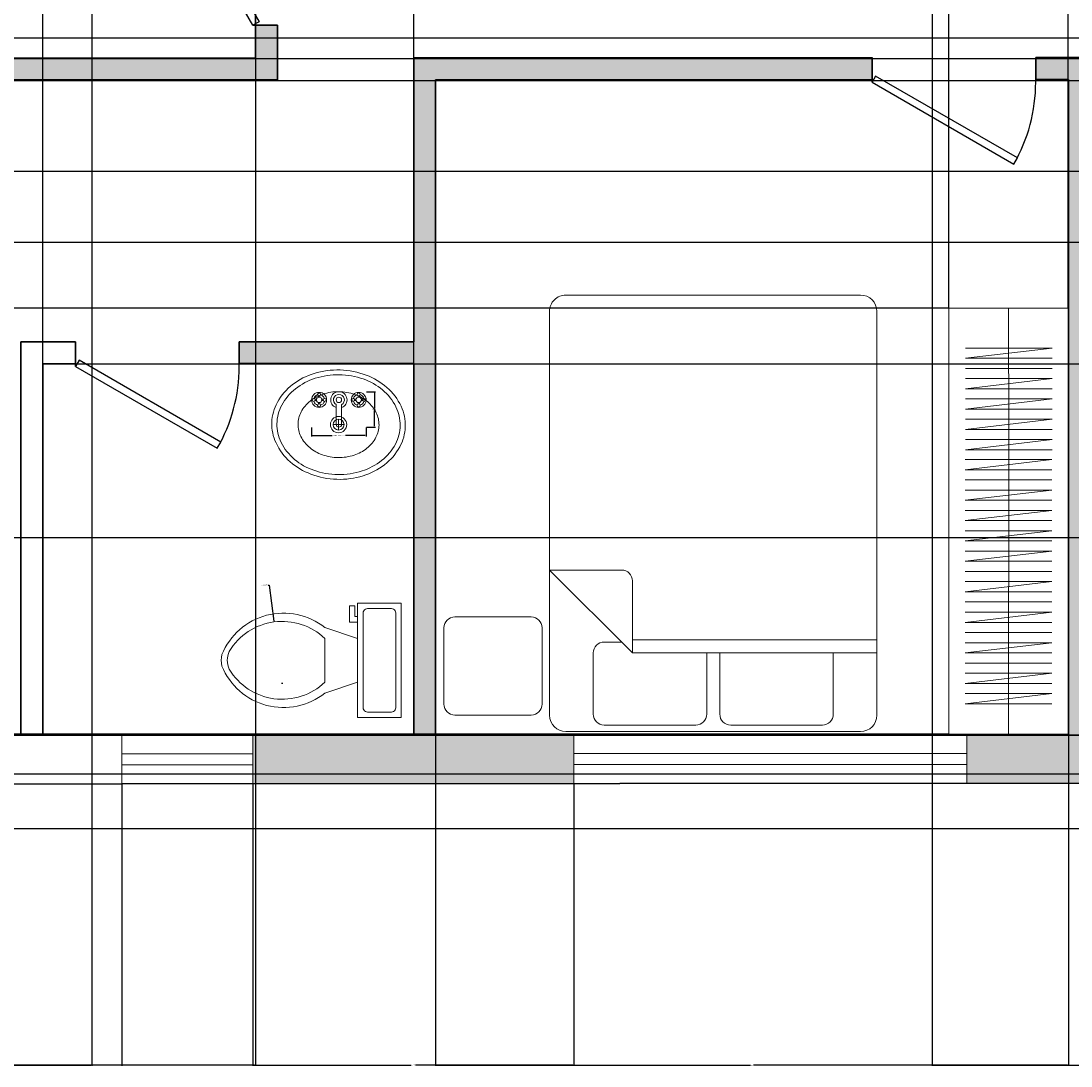
# Model space of a CAD drawing. Units: inches. Extents: x 1531 to 2263, y 2711 to 3216.
# Tile 2 of 12: x 1733 to 1925, y 2711 to 2903. Entities that reach past the tile are written whole.
import ezdxf

# ---------------------------------------------------------------- set-up
doc = ezdxf.new("R2010")
doc.units = ezdxf.units.IN
for name, color, linetype, lineweight in [('A-ANNO-DIMS', 2, 'Continuous', 18), ('A-DOOR', 3, 'Continuous', 25), ('A-FLOR-CASE', 9, 'Continuous', 18), ('A-FLOR-FIXT', 9, 'Continuous', 18), ('A-FURN', 8, 'Continuous', 18), ('A-GLAZ', 4, 'Continuous', 18), ('A-WALL', 7, 'Continuous', 35)]:
    doc.layers.add(name, color=color, linetype=linetype, lineweight=lineweight)
doc.layers.add('A-WALL-PATT', color=18, linetype='Continuous', lineweight=13, true_color=0x000000)
doc.styles.get("Standard").update_dxf_attribs({"font": 'arial.ttf'})
doc.dimstyles.get("Standard").update_dxf_attribs({"dimtxt": 0.18, "dimasz": 0.18, "dimexe": 0.18, "dimexo": 0.0625, "dimgap": 0.09, "dimtad": 0, "dimtih": 1, "dimtoh": 1, "dimdec": 4, "dimzin": 0, "dimdsep": 46, "dimtxsty": 'Standard', "dimcen": 0.09, "dimadec": 0, "dimazin": 0, "dimtfac": 1, "dimtdec": 4, "dimtofl": 0, "dimtmove": 0, "dimatfit": 3, "dimfxl": 1, "dimtolj": 1, "dimtzin": 0, "dimarcsym": 0})

# ---------------------------------------------------------------- blocks, each defined once
blk = doc.blocks.new('*U6')
for p, q in [((0, 0), (0, 6)), ((40, 0), (40, 6))]:
    blk.add_line(p, q)
blk.add_lwpolyline([(0, 0), (34.64, -20), (35.52, -18.48), (0.87, 1.52)], close=True)
blk.add_arc((0, 0), 40, 330, 0)
blk = doc.blocks.new('*U4')
for p, q in [((-40, 0), (-40, 6)), ((0, 0), (0, 6))]:
    blk.add_line(p, q)
blk.add_lwpolyline([(0, 0), (-34.64, -20), (-35.52, -18.48), (-0.88, 1.52)], close=True)
blk.add_arc((0, 0), 40, 180, 210)
blk = doc.blocks.new('Bed - Queen')
for p, q in [((3, 0), (57, 0)), ((10, -1.2), (26.8, -1.2)), ((33.2, -1.2), (50, -1.2)), ((0, -77), (0, -3)), ((8, -14.4), (8, -3.2)), ((28.8, -3.2), (28.8, -14.4)), ((31.2, -14.4), (31.2, -3.2)), ((52, -3.2), (52, -14.4)), ((60, -3), (60, -77)), ((0, -14.4), (44.8, -14.4)), ((60, -29.6), (44.8, -14.4)), ((44.8, -14.4), (44.8, -27.6)), ((44.8, -16.8), (0, -16.8)), ((50, -16.4), (46.8, -16.4)), ((46.8, -29.6), (60, -29.6)), ((57, -80), (3, -80))]:
    blk.add_line(p, q)
blk.add_lwpolyline([(63.37, -3.02), (77.37, -3.02, -0.414214), (79.37, -5.02), (79.37, -19.02, -0.414214), (77.37, -21.02), (63.37, -21.02, -0.414214), (61.37, -19.02), (61.37, -5.02, -0.414214)], format="xyb", close=True)
for centre, radius, start, end in [((3, -3), 3, 90, 180), ((57, -3), 3, 0, 90), ((10, -3.2), 2, 90, 180), ((26.8, -3.2), 2, 0, 90), ((33.2, -3.2), 2, 90, 180), ((50, -3.2), 2, 0, 90), ((50, -14.4), 2, 270, 0), ((46.8, -27.6), 2, 180, 270), ((3, -77), 3, 180, 270), ((57, -77), 3, 270, 0)]:
    blk.add_arc(centre, radius, start, end)
blk = doc.blocks.new('Toilet - top')
for p, q in [((9.5, -6), (9.5, -2)), ((-10, -8.5), (-8, -8.5)), ((-10, -9.5), (-10, -8.5)), ((-7, -9.5), (-10, -9.5)), ((-8, -8.5), (-8, -8)), ((-7, -8), (-7, -9.5)), ((-4, -8), (-6, -14)), ((4, -8), (6, -14)), ((4, -14), (-4, -14))]:
    blk.add_line(p, q)
blk.add_lwpolyline([(10.5, -8), (10.5, 0), (-10.5, 0), (-10.5, -8)], close=True)
for points in [[(8.5, -1), (-8.5, -1)], [(-9.5, -2), (-9.5, -6)], [(-8.5, -7), (8.5, -7)]]:
    blk.add_lwpolyline(points)
for centre, radius, start, end in [((-8.62, -1.88), 0.884, 81.8699, 188.1301), ((8.62, -1.88), 0.884, 351.8699, 98.1301), ((-8.62, -6.12), 0.884, 171.8699, 278.1301), ((8.62, -6.12), 0.884, 261.8699, 8.1301), ((3.52, -21.58), 12.17, 141.4691, 247.9714), ((4.2, -21.82), 11.33, 136.3677, 238.9468), ((-3.52, -21.58), 12.17, 292.0284, 38.5307), ((-4.2, -21.82), 11.33, 301.053, 43.6321), ((0, -27.88), 4, 245.7318, 294.2682), ((0, -29), 4, 254.8605, 285.1395)]:
    blk.add_arc(centre, radius, start, end)
blk = doc.blocks.new('Sink - Oval top')
for p, q in [((-1, 0), (1, 0)), ((0, 1), (0, -1))]:
    blk.add_line(p, q)
for points in [[(-12.23, 0.39, 0.117634), (-11.46, -3.36, 0.104469), (-8.88, -6.8, 0.090016), (-5.08, -9.07, 0.08192), (-0.32, -10.02, 0.08192), (4.49, -9.38, 0.090016), (8.42, -7.36, 0.104469), (11.22, -4.09, 0.117634), (12.23, -0.39, 0.117634), (11.46, 3.36, 0.104469), (8.88, 6.8, 0.090016), (5.08, 9.07, 0.08192), (0.32, 10.02, 0.08192), (-4.49, 9.38, 0.090016), (-8.42, 7.36, 0.104469), (-11.22, 4.09, 0.117634)], [(-11.29, 0.16, 0.118622), (-10.52, -3.25, 0.104678), (-8.07, -6.36, 0.089562), (-4.54, -8.37, 0.081185), (-0.13, -9.15, 0.081185), (4.3, -8.49, 0.089562), (7.89, -6.58, 0.104678), (10.42, -3.55, 0.118622), (11.29, -0.16, 0.118622), (10.52, 3.25, 0.104678), (8.07, 6.36, 0.089562), (4.54, 8.37, 0.081185), (0.13, 9.15, 0.081185), (-4.3, 8.49, 0.089562), (-7.89, 6.58, 0.104678), (-10.42, 3.55, 0.118622)], [(-7.42, 0.08, 0.118283), (-6.91, -2.17, 0.104607), (-5.29, -4.21, 0.089718), (-2.97, -5.53, 0.081436), (-0.07, -6.04, 0.081436), (2.84, -5.59, 0.089718), (5.2, -4.33, 0.104607), (6.86, -2.32, 0.118283), (7.42, -0.08, 0.118283), (6.91, 2.17, 0.104607), (5.29, 4.21, 0.089718), (2.97, 5.53, 0.081436), (0.07, 6.04, 0.081436), (-2.84, 5.59, 0.089718), (-5.2, 4.33, 0.104607), (-6.86, 2.32, 0.118283)]]:
    blk.add_lwpolyline(points, format="xyb", close=True)
for radius in [1.5, 1]:
    blk.add_circle((0, 0), radius)
blk = doc.blocks.new('Faucet - Bathroom top')
for p, q in [((-4.107, 0.125), (-4.375, 0.125)), ((-3.75, 0.4788), (-3.75, 0.75)), ((-3.5, 0.482), (-3.5, 0.75)), ((-3.1461, 0.125), (-2.875, 0.125)), ((3.143, 0.125), (2.875, 0.125)), ((3.5, 0.4788), (3.5, 0.75)), ((3.75, 0.482), (3.75, 0.75)), ((4.1039, 0.125), (4.375, 0.125)), ((-4.1039, -0.125), (-4.375, -0.125)), ((-3.75, -0.4821), (-3.75, -0.75)), ((-3.5, -0.4789), (-3.5, -0.75)), ((-3.143, -0.125), (-2.875, -0.125)), ((-0.5, -0.8639), (-0.5, -4.5)), ((0.5, -4.5), (0.5, -0.8631)), ((3.1461, -0.125), (2.875, -0.125)), ((3.5, -0.4821), (3.5, -0.75)), ((3.75, -0.4789), (3.75, -0.75)), ((4.107, -0.125), (4.375, -0.125))]:
    blk.add_line(p, q)
for centre, radius in [((-3.625, 0), 1.375), ((-4.625, 0), 0.2795), ((-3.625, 0), 0.5), ((-3.625, 1), 0.2795), ((-2.625, 0), 0.2795), ((0, 0), 0.5), ((3.625, 0), 1.375), ((2.625, 0), 0.2795), ((3.625, 0), 0.5), ((3.625, 1), 0.2795), ((4.625, 0), 0.2795), ((-3.625, -1), 0.2795), ((3.625, -1), 0.2795)]:
    blk.add_circle(centre, radius)
for centre, radius, start, end in [((-3.625, 0), 1, 105.2407, 164.2093), ((-3.625, 0), 1, 16.44125, 74.07887), ((0, 0), 1.5, 289.6514, 250.3603), ((0, 0), 1, 300.3431, 239.7554), ((3.625, 0), 1, 106.12, 164.0884), ((3.625, 0), 1, 16.23422, 73.90469), ((-3.625, 0), 1, 196.2342, 253.9047), ((-3.625, 0), 1, 286.12, 344.0884), ((3.625, 0), 1, 196.4413, 254.0789), ((3.625, 0), 1, 285.2407, 344.2093), ((0, -4.5), 0.5, 180, 0)]:
    blk.add_arc(centre, radius, start, end)
blk = doc.blocks.new('WIN-72IN')
for p, q in [((0, 5.5), (72, 5.5)), ((0, 3.5), (72, 3.5))]:
    blk.add_line(p, q)
for points in [[(0, 9), (0, 0)], [(72, 0), (72, 9)]]:
    blk.add_lwpolyline(points)
blk = doc.blocks.new('WIN-24IN')
for p, q in [((0, 5.5), (24, 5.5)), ((0, 3.5), (24, 3.5))]:
    blk.add_line(p, q)
for points in [[(0, 9), (0, 0)], [(24, 0), (24, 9)]]:
    blk.add_lwpolyline(points)
blk = doc.blocks.new('*D40')
at = {"layer": 'A-ANNO-DIMS', "color": 0, "lineweight": -2, "transparency": 16777216}
for p, q in [((1786.18, 2828.07), (1786.18, 2826.45)), ((1796.18, 2828.07), (1796.18, 2826.45)), ((1786.36, 2826.63), (1789.97, 2826.63)), ((1796, 2826.63), (1792.4, 2826.63))]:
    blk.add_line(p, q, dxfattribs=at)
at = {"layer": 'A-ANNO-DIMS', "color": 0, "transparency": 16777216}
for points in [[(1786.36, 2826.66), (1786.36, 2826.6), (1786.18, 2826.63)], [(1796, 2826.66), (1796, 2826.6), (1796.18, 2826.63)]]:
    blk.add_solid(points, dxfattribs=at)
at = {"layer": 'Defpoints', "color": 0, "transparency": 16777216}
for p in [(1786.18, 2828.13), (1796.18, 2828.13), (1796.18, 2826.63)]:
    blk.add_point(p, dxfattribs=at)
at = {"layer": 'A-ANNO-DIMS', "color": 0, "transparency": 16777216, "insert": (1791.18, 2826.63), "char_height": 0.18, "attachment_point": 5}
blk.add_mtext('\\A1;BASIN TAP 10 TYP.', dxfattribs=at)
blk = doc.blocks.new('*D41')
at = {"layer": 'A-ANNO-DIMS', "color": 0, "lineweight": -2, "transparency": 16777216}
for p, q in [((1796.25, 2834.63), (1797.86, 2834.63)), ((1797.68, 2834.45), (1797.68, 2831.56)), ((1797.68, 2828.31), (1797.68, 2831.2)), ((1796.25, 2828.13), (1797.86, 2828.13))]:
    blk.add_line(p, q, dxfattribs=at)
at = {"layer": 'A-ANNO-DIMS', "color": 0, "transparency": 16777216}
for points in [[(1797.65, 2834.45), (1797.71, 2834.45), (1797.68, 2834.63)], [(1797.65, 2828.31), (1797.71, 2828.31), (1797.68, 2828.13)]]:
    blk.add_solid(points, dxfattribs=at)
at = {"layer": 'Defpoints', "color": 0, "transparency": 16777216}
for p in [(1796.18, 2834.63), (1797.68, 2834.63), (1796.18, 2828.13)]:
    blk.add_point(p, dxfattribs=at)
at = {"layer": 'A-ANNO-DIMS', "color": 0, "transparency": 16777216, "insert": (1797.68, 2831.38), "char_height": 0.18, "attachment_point": 5}
blk.add_mtext('\\A1;7 TYP.', dxfattribs=at)
blk = doc.blocks.new('*D58')
at = {"layer": 'A-ANNO-DIMS', "color": 0, "lineweight": -2, "transparency": 16777216}
for p, q in [((1715.91, 3097.69), (1715.91, 2711.06)), ((1775.91, 3097.72), (1775.91, 2711.06)), ((1716.09, 2711.24), (1745.69, 2711.24)), ((1775.73, 2711.24), (1746.13, 2711.24))]:
    blk.add_line(p, q, dxfattribs=at)
at = {"layer": 'A-ANNO-DIMS', "color": 0, "transparency": 16777216}
for points in [[(1716.09, 2711.27), (1716.09, 2711.21), (1715.91, 2711.24)], [(1775.73, 2711.27), (1775.73, 2711.21), (1775.91, 2711.24)]]:
    blk.add_solid(points, dxfattribs=at)
at = {"layer": 'Defpoints', "color": 0, "transparency": 16777216}
for p in [(1715.91, 3097.75), (1775.91, 3097.78), (1775.91, 2711.24)]:
    blk.add_point(p, dxfattribs=at)
at = {"layer": 'A-ANNO-DIMS', "color": 0, "transparency": 16777216, "insert": (1745.91, 2711.24), "char_height": 0.18, "attachment_point": 5}
blk.add_mtext('\\A1;60', dxfattribs=at)
blk = doc.blocks.new('*D60')
at = {"layer": 'A-ANNO-DIMS', "color": 0, "lineweight": -2, "transparency": 16777216}
for p, q in [((1899.91, 3097.79), (1899.91, 2711.06)), ((1955.91, 3097.81), (1955.91, 2711.06)), ((1900.09, 2711.24), (1927.69, 2711.24)), ((1955.73, 2711.24), (1928.13, 2711.24))]:
    blk.add_line(p, q, dxfattribs=at)
at = {"layer": 'A-ANNO-DIMS', "color": 0, "transparency": 16777216}
for points in [[(1900.09, 2711.27), (1900.09, 2711.21), (1899.91, 2711.24)], [(1955.73, 2711.27), (1955.73, 2711.21), (1955.91, 2711.24)]]:
    blk.add_solid(points, dxfattribs=at)
at = {"layer": 'Defpoints', "color": 0, "transparency": 16777216}
for p in [(1899.91, 3097.85), (1955.91, 3097.88), (1955.91, 2711.24)]:
    blk.add_point(p, dxfattribs=at)
at = {"layer": 'A-ANNO-DIMS', "color": 0, "transparency": 16777216, "insert": (1927.91, 2711.24), "char_height": 0.18, "attachment_point": 5}
blk.add_mtext('\\A1;56', dxfattribs=at)
blk = doc.blocks.new('*D64')
at = {"layer": 'A-ANNO-DIMS', "color": 0, "lineweight": -2, "transparency": 16777216}
for p, q in [((1779.85, 3025.79), (1531.04, 3025.79)), ((1531.22, 3025.61), (1531.22, 2960.97)), ((1531.22, 2895.96), (1531.22, 2960.6)), ((1775.85, 2895.78), (1531.04, 2895.78))]:
    blk.add_line(p, q, dxfattribs=at)
at = {"layer": 'A-ANNO-DIMS', "color": 0, "transparency": 16777216}
for points in [[(1531.19, 3025.61), (1531.25, 3025.61), (1531.22, 3025.79)], [(1531.19, 2895.96), (1531.25, 2895.96), (1531.22, 2895.78)]]:
    blk.add_solid(points, dxfattribs=at)
at = {"layer": 'Defpoints', "color": 0, "transparency": 16777216}
for p in [(1779.91, 3025.79), (1531.22, 2895.78), (1775.91, 2895.78)]:
    blk.add_point(p, dxfattribs=at)
at = {"layer": 'A-ANNO-DIMS', "color": 0, "transparency": 16777216, "insert": (1531.22, 2960.78), "char_height": 0.18, "attachment_point": 5}
blk.add_mtext('\\A1;130', dxfattribs=at)
blk = doc.blocks.new('*D65')
at = {"layer": 'A-ANNO-DIMS', "color": 0, "lineweight": -2, "transparency": 16777216}
for p, q in [((1577.97, 2891.68), (2262.37, 2891.68)), ((2262.19, 2891.5), (2262.19, 2831.86)), ((2262.19, 2771.86), (2262.19, 2831.5)), ((1577.97, 2771.68), (2262.37, 2771.68))]:
    blk.add_line(p, q, dxfattribs=at)
at = {"layer": 'A-ANNO-DIMS', "color": 0, "transparency": 16777216}
for points in [[(2262.16, 2891.5), (2262.22, 2891.5), (2262.19, 2891.68)], [(2262.16, 2771.86), (2262.22, 2771.86), (2262.19, 2771.68)]]:
    blk.add_solid(points, dxfattribs=at)
at = {"layer": 'Defpoints', "color": 0, "transparency": 16777216}
for p in [(1577.91, 2891.68), (1577.91, 2771.68), (2262.19, 2771.68)]:
    blk.add_point(p, dxfattribs=at)
at = {"layer": 'A-ANNO-DIMS', "color": 0, "transparency": 16777216, "insert": (2262.19, 2831.68), "char_height": 0.18, "attachment_point": 5}
blk.add_mtext('\\A1;120', dxfattribs=at)
blk = doc.blocks.new('*D66')
at = {"layer": 'A-ANNO-DIMS', "color": 0, "lineweight": -2, "transparency": 16777216}
for p, q in [((1577.91, 2895.74), (1577.91, 3216.47)), ((1578.09, 3216.29), (1676.63, 3216.29)), ((1775.73, 3216.29), (1677.19, 3216.29)), ((1775.91, 2895.85), (1775.91, 3216.47))]:
    blk.add_line(p, q, dxfattribs=at)
at = {"layer": 'A-ANNO-DIMS', "color": 0, "transparency": 16777216}
for points in [[(1578.09, 3216.32), (1578.09, 3216.26), (1577.91, 3216.29)], [(1775.73, 3216.32), (1775.73, 3216.26), (1775.91, 3216.29)]]:
    blk.add_solid(points, dxfattribs=at)
at = {"layer": 'Defpoints', "color": 0, "transparency": 16777216}
for p in [(1775.91, 3216.29), (1577.91, 2895.68), (1775.91, 2895.78)]:
    blk.add_point(p, dxfattribs=at)
at = {"layer": 'A-ANNO-DIMS', "color": 0, "transparency": 16777216, "insert": (1676.91, 3216.29), "char_height": 0.18, "attachment_point": 5}
blk.add_mtext('\\A1;198', dxfattribs=at)
blk = doc.blocks.new('*D68')
at = {"layer": 'A-ANNO-DIMS', "color": 0, "lineweight": -2, "transparency": 16777216}
for p, q in [((1736.91, 2839.83), (1736.91, 3216.47)), ((1737.09, 3216.29), (1770.69, 3216.29)), ((1804.73, 3216.29), (1771.13, 3216.29)), ((1804.91, 2839.86), (1804.91, 3216.47))]:
    blk.add_line(p, q, dxfattribs=at)
at = {"layer": 'A-ANNO-DIMS', "color": 0, "transparency": 16777216}
for points in [[(1737.09, 3216.32), (1737.09, 3216.26), (1736.91, 3216.29)], [(1804.73, 3216.32), (1804.73, 3216.26), (1804.91, 3216.29)]]:
    blk.add_solid(points, dxfattribs=at)
at = {"layer": 'Defpoints', "color": 0, "transparency": 16777216}
for p in [(1804.91, 3216.29), (1736.91, 2839.76), (1804.91, 2839.8)]:
    blk.add_point(p, dxfattribs=at)
at = {"layer": 'A-ANNO-DIMS', "color": 0, "transparency": 16777216, "insert": (1770.91, 3216.29), "char_height": 0.18, "attachment_point": 5}
blk.add_mtext('\\A1;68', dxfattribs=at)
blk = doc.blocks.new('*D69')
at = {"layer": 'A-ANNO-DIMS', "color": 0, "lineweight": -2, "transparency": 16777216}
for p, q in [((1808.91, 2891.74), (1808.91, 2711.06)), ((1924.91, 2891.8), (1924.91, 2711.06)), ((1809.09, 2711.24), (1866.63, 2711.24)), ((1924.73, 2711.24), (1867.19, 2711.24))]:
    blk.add_line(p, q, dxfattribs=at)
at = {"layer": 'A-ANNO-DIMS', "color": 0, "transparency": 16777216}
for points in [[(1809.09, 2711.27), (1809.09, 2711.21), (1808.91, 2711.24)], [(1924.73, 2711.27), (1924.73, 2711.21), (1924.91, 2711.24)]]:
    blk.add_solid(points, dxfattribs=at)
at = {"layer": 'Defpoints', "color": 0, "transparency": 16777216}
for p in [(1808.91, 2891.8), (1924.91, 2891.86), (1924.91, 2711.24)]:
    blk.add_point(p, dxfattribs=at)
at = {"layer": 'A-ANNO-DIMS', "color": 0, "transparency": 16777216, "insert": (1866.91, 2711.24), "char_height": 0.18, "attachment_point": 5}
blk.add_mtext('\\A1;116', dxfattribs=at)
blk = doc.blocks.new('*D70')
at = {"layer": 'A-ANNO-DIMS', "color": 0, "lineweight": -2, "transparency": 16777216}
for p, q in [((1736.97, 2839.76), (2262.37, 2839.76)), ((2262.19, 2839.58), (2262.19, 2805.94)), ((2262.19, 2771.94), (2262.19, 2805.58)), ((1736.97, 2771.76), (2262.37, 2771.76))]:
    blk.add_line(p, q, dxfattribs=at)
at = {"layer": 'A-ANNO-DIMS', "color": 0, "transparency": 16777216}
for points in [[(2262.16, 2839.58), (2262.22, 2839.58), (2262.19, 2839.76)], [(2262.16, 2771.94), (2262.22, 2771.94), (2262.19, 2771.76)]]:
    blk.add_solid(points, dxfattribs=at)
at = {"layer": 'Defpoints', "color": 0, "transparency": 16777216}
for p in [(1736.91, 2839.76), (2262.19, 2839.76), (1736.91, 2771.76)]:
    blk.add_point(p, dxfattribs=at)
at = {"layer": 'A-ANNO-DIMS', "color": 0, "transparency": 16777216, "insert": (2262.19, 2805.76), "char_height": 0.18, "attachment_point": 5}
blk.add_mtext('\\A1;68', dxfattribs=at)
blk = doc.blocks.new('*D75')
at = {"layer": 'A-ANNO-DIMS', "color": 0, "lineweight": -2, "transparency": 16777216}
for p, q in [((2219.85, 2899.4), (1531.04, 2899.4)), ((1531.22, 2899.22), (1531.22, 2853.81)), ((1531.22, 2808.04), (1531.22, 2853.45)), ((2219.85, 2807.86), (1531.04, 2807.86))]:
    blk.add_line(p, q, dxfattribs=at)
at = {"layer": 'A-ANNO-DIMS', "color": 0, "transparency": 16777216}
for points in [[(1531.19, 2899.22), (1531.25, 2899.22), (1531.22, 2899.4)], [(1531.19, 2808.04), (1531.25, 2808.04), (1531.22, 2807.86)]]:
    blk.add_solid(points, dxfattribs=at)
at = {"layer": 'Defpoints', "color": 0, "transparency": 16777216}
for p in [(1531.22, 2899.4), (2219.91, 2899.4), (2219.91, 2807.86)]:
    blk.add_point(p, dxfattribs=at)
at = {"layer": 'A-ANNO-DIMS', "color": 0, "transparency": 16777216, "insert": (1531.22, 2853.63), "char_height": 0.18, "attachment_point": 5}
blk.add_mtext('\\A1;91.53', dxfattribs=at)
blk = doc.blocks.new('*D87')
at = {"layer": 'A-ANNO-DIMS', "color": 0, "lineweight": -2, "transparency": 16777216}
for p, q in [((1721.91, 3101.69), (1721.91, 2711.06)), ((1745.91, 3101.7), (1745.91, 2711.06)), ((1722.09, 2711.24), (1733.69, 2711.24)), ((1745.73, 2711.24), (1734.13, 2711.24))]:
    blk.add_line(p, q, dxfattribs=at)
at = {"layer": 'A-ANNO-DIMS', "color": 0, "transparency": 16777216}
for points in [[(1722.09, 2711.27), (1722.09, 2711.21), (1721.91, 2711.24)], [(1745.73, 2711.27), (1745.73, 2711.21), (1745.91, 2711.24)]]:
    blk.add_solid(points, dxfattribs=at)
at = {"layer": 'Defpoints', "color": 0, "transparency": 16777216}
for p in [(1721.91, 3101.75), (1745.91, 3101.77), (1745.91, 2711.24)]:
    blk.add_point(p, dxfattribs=at)
at = {"layer": 'A-ANNO-DIMS', "color": 0, "transparency": 16777216, "insert": (1733.91, 2711.24), "char_height": 0.18, "attachment_point": 5}
blk.add_mtext('\\A1;24', dxfattribs=at)
blk = doc.blocks.new('*D94')
at = {"layer": 'A-ANNO-DIMS', "color": 0, "lineweight": -2, "transparency": 16777216}
for p, q in [((1693.26, 2762.64), (1693.26, 2711.06)), ((1751.41, 2762.71), (1751.41, 2711.06)), ((1693.44, 2711.24), (1721.94, 2711.24)), ((1751.23, 2711.24), (1722.73, 2711.24))]:
    blk.add_line(p, q, dxfattribs=at)
at = {"layer": 'A-ANNO-DIMS', "color": 0, "transparency": 16777216}
for points in [[(1693.44, 2711.27), (1693.44, 2711.21), (1693.26, 2711.24)], [(1751.23, 2711.27), (1751.23, 2711.21), (1751.41, 2711.24)]]:
    blk.add_solid(points, dxfattribs=at)
at = {"layer": 'Defpoints', "color": 0, "transparency": 16777216}
for p in [(1693.26, 2762.7), (1751.41, 2762.77), (1751.41, 2711.24)]:
    blk.add_point(p, dxfattribs=at)
at = {"layer": 'A-ANNO-DIMS', "color": 0, "transparency": 16777216, "insert": (1722.34, 2711.24), "char_height": 0.18, "attachment_point": 5}
blk.add_mtext('\\A1;58.15', dxfattribs=at)
blk = doc.blocks.new('*D95')
at = {"layer": 'A-ANNO-DIMS', "color": 0, "lineweight": -2, "transparency": 16777216}
for p, q in [((1775.41, 2762.71), (1775.41, 2711.06)), ((1834.26, 2762.75), (1834.26, 2711.06)), ((1775.59, 2711.24), (1804.44, 2711.24)), ((1834.08, 2711.24), (1805.23, 2711.24))]:
    blk.add_line(p, q, dxfattribs=at)
at = {"layer": 'A-ANNO-DIMS', "color": 0, "transparency": 16777216}
for points in [[(1775.59, 2711.27), (1775.59, 2711.21), (1775.41, 2711.24)], [(1834.08, 2711.27), (1834.08, 2711.21), (1834.26, 2711.24)]]:
    blk.add_solid(points, dxfattribs=at)
at = {"layer": 'Defpoints', "color": 0, "transparency": 16777216}
for p in [(1775.41, 2762.77), (1834.26, 2762.81), (1834.26, 2711.24)]:
    blk.add_point(p, dxfattribs=at)
at = {"layer": 'A-ANNO-DIMS', "color": 0, "transparency": 16777216, "insert": (1804.84, 2711.24), "char_height": 0.18, "attachment_point": 5}
blk.add_mtext('\\A1;58.85', dxfattribs=at)
blk = doc.blocks.new('*D101')
at = {"layer": 'A-ANNO-DIMS', "color": 0, "lineweight": -2, "transparency": 16777216}
for p, q in [((2228.85, 2918.81), (1531.04, 2918.81)), ((1531.22, 2918.63), (1531.22, 2897.08)), ((1531.22, 2875.18), (1531.22, 2896.72)), ((2228.85, 2875), (1531.04, 2875))]:
    blk.add_line(p, q, dxfattribs=at)
at = {"layer": 'A-ANNO-DIMS', "color": 0, "transparency": 16777216}
for points in [[(1531.19, 2918.63), (1531.25, 2918.63), (1531.22, 2918.81)], [(1531.19, 2875.18), (1531.25, 2875.18), (1531.22, 2875)]]:
    blk.add_solid(points, dxfattribs=at)
at = {"layer": 'Defpoints', "color": 0, "transparency": 16777216}
for p in [(2228.91, 2918.81), (1531.22, 2875), (2228.91, 2875)]:
    blk.add_point(p, dxfattribs=at)
at = {"layer": 'A-ANNO-DIMS', "color": 0, "transparency": 16777216, "insert": (1531.22, 2896.9), "char_height": 0.18, "attachment_point": 5}
blk.add_mtext('\\A1;43.81', dxfattribs=at)
blk = doc.blocks.new('*D114')
at = {"layer": 'A-ANNO-DIMS', "color": 0, "lineweight": -2, "transparency": 16777216}
for p, q in [((1577.97, 2913.94), (2262.37, 2913.94)), ((2262.19, 2913.76), (2262.19, 2904.99)), ((2262.19, 2895.86), (2262.19, 2904.63)), ((1577.97, 2895.68), (2262.37, 2895.68))]:
    blk.add_line(p, q, dxfattribs=at)
at = {"layer": 'A-ANNO-DIMS', "color": 0, "transparency": 16777216}
for points in [[(2262.16, 2913.76), (2262.22, 2913.76), (2262.19, 2913.94)], [(2262.16, 2895.86), (2262.22, 2895.86), (2262.19, 2895.68)]]:
    blk.add_solid(points, dxfattribs=at)
at = {"layer": 'Defpoints', "color": 0, "transparency": 16777216}
for p in [(1577.91, 2913.94), (1577.91, 2895.68), (2262.19, 2895.68)]:
    blk.add_point(p, dxfattribs=at)
at = {"layer": 'A-ANNO-DIMS', "color": 0, "transparency": 16777216, "insert": (2262.19, 2904.81), "char_height": 0.18, "attachment_point": 5}
blk.add_mtext('\\A1;18.26', dxfattribs=at)
blk = doc.blocks.new('*D125')
at = {"layer": 'A-ANNO-DIMS', "color": 0, "lineweight": -2, "transparency": 16777216}
for p, q in [((2076.85, 2861.95), (1531.04, 2861.95)), ((1531.22, 2861.77), (1531.22, 2835.09)), ((1531.22, 2808.04), (1531.22, 2834.72)), ((2076.85, 2807.86), (1531.04, 2807.86))]:
    blk.add_line(p, q, dxfattribs=at)
at = {"layer": 'A-ANNO-DIMS', "color": 0, "transparency": 16777216}
for points in [[(1531.19, 2861.77), (1531.25, 2861.77), (1531.22, 2861.95)], [(1531.19, 2808.04), (1531.25, 2808.04), (1531.22, 2807.86)]]:
    blk.add_solid(points, dxfattribs=at)
at = {"layer": 'Defpoints', "color": 0, "transparency": 16777216}
for p in [(2076.91, 2861.95), (1531.22, 2807.86), (2076.91, 2807.86)]:
    blk.add_point(p, dxfattribs=at)
at = {"layer": 'A-ANNO-DIMS', "color": 0, "transparency": 16777216, "insert": (1531.22, 2834.91), "char_height": 0.18, "attachment_point": 5}
blk.add_mtext('\\A1;54.09', dxfattribs=at)
blk = doc.blocks.new('*D126')
at = {"layer": 'A-ANNO-DIMS', "color": 0, "lineweight": -2, "transparency": 16777216}
for p, q in [((1902.99, 2850), (1902.99, 3216.47)), ((1903.17, 3216.29), (1913.45, 3216.29)), ((1924.67, 3216.29), (1914.38, 3216.29)), ((1924.85, 2850), (1924.85, 3216.47))]:
    blk.add_line(p, q, dxfattribs=at)
at = {"layer": 'A-ANNO-DIMS', "color": 0, "transparency": 16777216}
for points in [[(1903.17, 3216.32), (1903.17, 3216.26), (1902.99, 3216.29)], [(1924.67, 3216.32), (1924.67, 3216.26), (1924.85, 3216.29)]]:
    blk.add_solid(points, dxfattribs=at)
at = {"layer": 'Defpoints', "color": 0, "transparency": 16777216}
for p in [(1924.85, 3216.29), (1902.99, 2849.94), (1924.85, 2849.94)]:
    blk.add_point(p, dxfattribs=at)
at = {"layer": 'A-ANNO-DIMS', "color": 0, "transparency": 16777216, "insert": (1913.92, 3216.29), "char_height": 0.18, "attachment_point": 5}
blk.add_mtext('\\A1;21.866', dxfattribs=at)
blk = doc.blocks.new('*D127')
at = {"layer": 'A-ANNO-DIMS', "color": 0, "lineweight": -2, "transparency": 16777216}
for p, q in [((1902.92, 2849.94), (1531.04, 2849.94)), ((1531.22, 2849.76), (1531.22, 2811.07)), ((1531.22, 2772.03), (1531.22, 2810.71)), ((1902.92, 2771.85), (1531.04, 2771.85))]:
    blk.add_line(p, q, dxfattribs=at)
at = {"layer": 'A-ANNO-DIMS', "color": 0, "transparency": 16777216}
for points in [[(1531.19, 2849.76), (1531.25, 2849.76), (1531.22, 2849.94)], [(1531.19, 2772.03), (1531.25, 2772.03), (1531.22, 2771.85)]]:
    blk.add_solid(points, dxfattribs=at)
at = {"layer": 'Defpoints', "color": 0, "transparency": 16777216}
for p in [(1902.99, 2849.94), (1531.22, 2771.85), (1902.99, 2771.85)]:
    blk.add_point(p, dxfattribs=at)
at = {"layer": 'A-ANNO-DIMS', "color": 0, "transparency": 16777216, "insert": (1531.22, 2810.89), "char_height": 0.18, "attachment_point": 5}
blk.add_mtext('\\A1;78.09', dxfattribs=at)
blk = doc.blocks.new('*D131')
at = {"layer": 'A-ANNO-DIMS', "color": 0, "lineweight": -2, "transparency": 16777216}
for p, q in [((1986.59, 2764.52), (1531.04, 2764.52)), ((1531.22, 2764.34), (1531.22, 2759.7)), ((1531.22, 2754.7), (1531.22, 2759.33)), ((1986.59, 2754.52), (1531.04, 2754.52))]:
    blk.add_line(p, q, dxfattribs=at)
at = {"layer": 'A-ANNO-DIMS', "color": 0, "transparency": 16777216}
for points in [[(1531.19, 2764.34), (1531.25, 2764.34), (1531.22, 2764.52)], [(1531.19, 2754.7), (1531.25, 2754.7), (1531.22, 2754.52)]]:
    blk.add_solid(points, dxfattribs=at)
at = {"layer": 'Defpoints', "color": 0, "transparency": 16777216}
for p in [(1531.22, 2764.52), (1986.65, 2764.52), (1986.65, 2754.52)]:
    blk.add_point(p, dxfattribs=at)
at = {"layer": 'A-ANNO-DIMS', "color": 0, "transparency": 16777216, "insert": (1531.22, 2759.52), "char_height": 0.18, "attachment_point": 5}
blk.add_mtext('\\A1;10', dxfattribs=at)
blk = doc.blocks.new('*D133')
at = {"layer": 'A-ANNO-DIMS', "color": 0, "lineweight": -2, "transparency": 16777216}
for p, q in [((1778.2, 2799.17), (1778.38, 2799.17)), ((1778.38, 2799.17), (1779.26, 2792.61)), ((1780.7, 2781.21), (1780.88, 2781.21)), ((1780.79, 2781.12), (1780.79, 2781.3))]:
    blk.add_line(p, q, dxfattribs=at)
at = {"layer": 'A-ANNO-DIMS', "color": 0, "transparency": 16777216}
blk.add_solid([(1779.29, 2792.62), (1779.23, 2792.61), (1779.28, 2792.43)], dxfattribs=at)
at = {"layer": 'Defpoints', "color": 0, "transparency": 16777216}
for p in [(1779.28, 2792.43), (1780.79, 2781.21)]:
    blk.add_point(p, dxfattribs=at)
at = {"layer": 'A-ANNO-DIMS', "color": 0, "transparency": 16777216, "insert": (1777.53, 2799.17), "char_height": 0.18, "attachment_point": 5}
blk.add_mtext('\\A1;8X R11.33', dxfattribs=at)

msp = doc.modelspace()

# ---------------------------------------------------------------- hatches: boundary and pattern name
at = {"layer": 'A-WALL-PATT'}
h = msp.add_hatch(color=256, dxfattribs=at)
h.dxf.hatch_style = 1
h.paths.add_polyline_path([(1577.9111, 2891.6796), (1779.9101, 2891.7852), (1779.9101, 2895.7852), (1779.9101, 2901.7852), (1775.9101, 2901.7831), (1775.9101, 2895.7831), (1577.8462, 2895.6795), (1568.9111, 2895.6795), (1568.9111, 2840.9289), (1577.9111, 2840.9289)])
h = msp.add_hatch(color=256, dxfattribs=at)
h.dxf.hatch_style = 1
h.paths.add_polyline_path([(1834.2623, 2771.8136), (1808.9101, 2771.8004), (1808.9101, 2891.8004), (1888.9101, 2891.8422), (1888.9101, 2895.8422), (1804.9101, 2895.7983), (1804.9101, 2891.7983), (1804.9101, 2843.7983), (1772.9101, 2843.7815), (1772.9101, 2839.7815), (1804.9101, 2839.7983), (1804.9101, 2771.7983), (1775.4106, 2771.7828), (1775.4106, 2762.7828), (1834.2623, 2762.8136)])
h = msp.add_hatch(color=256, dxfattribs=at)
h.dxf.hatch_style = 1
h.paths.add_polyline_path([(1946.1667, 2807.8631), (1933.9101, 2807.8631), (1933.9101, 2891.8657), (1947.4101, 2891.8728), (1947.4101, 2895.4791), (1947.4101, 2895.8728), (1918.9101, 2895.8579), (1918.9101, 2891.861), (1924.9101, 2891.861), (1924.9101, 2771.8496), (1906.2623, 2771.8496), (1906.2623, 2762.8513), (1933.9101, 2762.8657), (1933.9101, 2771.861), (1933.9101, 2798.8631), (1937.9101, 2798.8631), (1946.1667, 2798.8631)])

# ---------------------------------------------------------------- linework, layer by layer
at = {"layer": 'A-FLOR-CASE'}
for p, q in [((1902.9862, 2849.9364), (1924.852, 2849.9364)), ((1902.9862, 2825.9364), (1902.9862, 2849.9364)), ((1913.9862, 2825.9364), (1913.9191, 2849.9364)), ((1906.0509, 2842.6379), (1921.9167, 2842.6379)), ((1921.9167, 2842.6379), (1906.0509, 2840.7728)), ((1906.0509, 2842.6379), (1921.9167, 2842.6379)), ((1921.9167, 2842.6379), (1906.0509, 2840.7728)), ((1906.0509, 2840.7728), (1921.9167, 2840.7728)), ((1906.0509, 2840.7728), (1921.9167, 2840.7728)), ((1906.0509, 2838.9076), (1921.9167, 2838.9076)), ((1906.0509, 2837.0425), (1921.9167, 2837.0425)), ((1921.9167, 2837.0425), (1906.0509, 2835.1774)), ((1906.0509, 2835.1774), (1921.9167, 2835.1774)), ((1906.0509, 2833.3122), (1921.9167, 2833.3122)), ((1921.9167, 2833.3122), (1906.0509, 2831.4471)), ((1906.0509, 2831.4471), (1921.9167, 2831.4471)), ((1906.0509, 2829.582), (1921.9167, 2829.582)), ((1921.9167, 2829.582), (1906.0509, 2827.7168)), ((1906.0509, 2827.7168), (1921.9167, 2827.7168)), ((1902.9862, 2825.9364), (1902.9862, 2771.8496)), ((1902.9862, 2771.8496), (1902.9862, 2825.9364)), ((1906.0509, 2825.8517), (1921.9167, 2825.8517)), ((1921.9167, 2825.8517), (1906.0509, 2823.9865)), ((1913.9862, 2825.9364), (1913.9191, 2771.8496)), ((1924.9862, 2825.9364), (1924.852, 2825.9364)), ((1924.852, 2825.9364), (1924.852, 2771.8496)), ((1924.9862, 2825.9385), (1925.0019, 2825.9385)), ((1902.9811, 2824.0713), (1902.9862, 2824.0713)), ((1906.0509, 2823.9865), (1921.9167, 2823.9865)), ((1902.9759, 2822.2061), (1902.9862, 2822.2061)), ((1905.9862, 2822.2061), (1921.852, 2822.2061)), ((1921.852, 2822.2061), (1905.9862, 2820.341)), ((1902.9707, 2820.341), (1902.9862, 2820.341)), ((1905.9862, 2820.341), (1921.852, 2820.341)), ((1905.9862, 2818.4758), (1921.852, 2818.4758)), ((1905.9862, 2816.6107), (1921.852, 2816.6107)), ((1921.852, 2816.6107), (1905.9862, 2814.7456)), ((1905.9862, 2814.7456), (1921.852, 2814.7456)), ((1905.9862, 2812.8804), (1921.852, 2812.8804)), ((1921.852, 2812.8804), (1905.9862, 2811.0153)), ((1905.9862, 2811.0153), (1921.852, 2811.0153)), ((1905.9862, 2809.1502), (1921.852, 2809.1502)), ((1921.852, 2809.1502), (1905.9862, 2807.285)), ((1905.9862, 2807.285), (1921.852, 2807.285)), ((1905.9862, 2805.4199), (1921.852, 2805.4199)), ((1921.852, 2805.4199), (1905.9862, 2803.5548)), ((1905.9862, 2803.5548), (1921.852, 2803.5548)), ((1905.9862, 2801.6896), (1921.852, 2801.6896)), ((1905.9862, 2799.8245), (1921.852, 2799.8245)), ((1921.852, 2799.8245), (1905.9862, 2797.9594)), ((1905.9862, 2797.9594), (1921.852, 2797.9594)), ((1905.9862, 2796.0942), (1921.852, 2796.0942)), ((1905.9862, 2794.2291), (1921.852, 2794.2291)), ((1921.852, 2794.2291), (1905.9862, 2792.364)), ((1905.9862, 2792.364), (1921.852, 2792.364)), ((1905.9862, 2790.4988), (1921.852, 2790.4988)), ((1905.9862, 2788.6337), (1921.852, 2788.6337)), ((1921.852, 2788.6337), (1905.9862, 2786.7685)), ((1905.9862, 2786.7685), (1921.852, 2786.7685)), ((1905.9862, 2784.9034), (1921.852, 2784.9034)), ((1905.9862, 2783.0383), (1921.852, 2783.0383)), ((1921.852, 2783.0383), (1905.9862, 2781.1731)), ((1905.9862, 2781.1731), (1921.852, 2781.1731)), ((1905.9862, 2779.308), (1921.852, 2779.308)), ((1921.852, 2779.308), (1905.9862, 2777.4429)), ((1905.9862, 2777.4429), (1921.852, 2777.4429)), ((1924.852, 2771.8496), (1902.9862, 2771.8496))]:
    msp.add_line(p, q, dxfattribs=at)
at = {"layer": 'A-WALL'}
for p, q in [((1779.9101, 2901.7852), (1775.907, 2901.7831)), ((1775.9101, 2901.7831), (1775.9101, 2895.7831)), ((1779.9101, 2901.7852), (1779.9101, 2895.7852)), ((1775.9101, 2895.7831), (1577.8462, 2895.6795)), ((1779.9101, 2895.7852), (1779.9101, 2891.7852)), ((1888.9101, 2895.8422), (1804.9101, 2895.7983)), ((1804.9101, 2891.7983), (1804.9101, 2895.7983)), ((1888.9101, 2891.8422), (1888.9101, 2895.861)), ((1947.4101, 2895.8728), (1918.9101, 2895.8579)), ((1918.9101, 2891.861), (1918.9101, 2895.861)), ((1779.9101, 2891.7852), (1577.8483, 2891.6795)), ((1732.9101, 2891.7983), (1732.9101, 2891.7606)), ((1804.9101, 2891.7983), (1804.9101, 2843.7983)), ((1888.9101, 2891.8422), (1808.9101, 2891.8004)), ((1808.9101, 2891.8004), (1808.9101, 2771.8004)), ((1918.9101, 2891.861), (1924.9101, 2891.861)), ((1924.9101, 2891.861), (1924.9101, 2771.861)), ((1924.9101, 2891.861), (1924.9101, 2771.861)), ((1742.9101, 2843.7659), (1732.9101, 2843.7606)), ((1732.9101, 2843.7606), (1732.9101, 2771.7606)), ((1742.9101, 2839.7627), (1742.9101, 2843.7659)), ((1804.9101, 2843.7983), (1772.9101, 2843.7815)), ((1772.9101, 2839.7627), (1772.9101, 2843.7815)), ((1742.9101, 2839.7659), (1736.9101, 2839.7627)), ((1736.9101, 2839.7627), (1736.9101, 2771.7627)), ((1804.9101, 2839.7983), (1772.9101, 2839.7815)), ((1804.9101, 2839.7983), (1804.9101, 2771.7983)), ((1924.9101, 2798.861), (1924.9101, 2771.861)), ((1732.9101, 2771.7606), (1577.9111, 2771.6796)), ((1804.9101, 2771.7983), (1736.9101, 2771.7627)), ((1924.9101, 2771.861), (1808.9101, 2771.8004))]:
    msp.add_line(p, q, dxfattribs=at)
msp.add_lwpolyline([(1933.9101, 2762.8657), (1568.9111, 2762.6748), (1568.9111, 3182.6749), (2228.9101, 3183.02), (2228.9101, 2798.8631)], dxfattribs=at)

# ---------------------------------------------------------------- block references
at = {"layer": 'A-DOOR', "xscale": 0.75, "yscale": 0.75, "zscale": 0.75, "rotation": 270}
msp.add_blockref('*U4', (1775.4101, 2901.7852), dxfattribs=at)
at = {"layer": 'A-DOOR', "xscale": 0.75, "yscale": 0.75, "zscale": 0.75}
for p in [(1888.9101, 2891.3422), (1742.9101, 2839.2659)]:
    msp.add_blockref('*U6', p, dxfattribs=at)
at = {"layer": 'A-FLOR-FIXT'}
for name, p in [('Sink - Oval top', (1791.116, 2828.5966)), ('Faucet - Bathroom top', (1791.1837, 2833.1334))]:
    msp.add_blockref(name, p, dxfattribs=at)
at = {"layer": 'A-FLOR-FIXT', "rotation": 270}
msp.add_blockref('Toilet - top', (1802.6105, 2785.4053), dxfattribs=at)
at = {"layer": 'A-FURN', "rotation": 180}
msp.add_blockref('Bed - Queen', (1889.7988, 2772.3501), dxfattribs=at)
at = {"layer": 'A-GLAZ'}
for name, p in [('WIN-24IN', (1751.4108, 2762.77)), ('WIN-72IN', (1834.2625, 2762.8136))]:
    msp.add_blockref(name, p, dxfattribs=at)

# ---------------------------------------------------------------- dimensions: what is measured, and where the dimension line sits
at = {"layer": 'A-ANNO-DIMS'}
for base, p1, p2, override, picture, middle in [((1775.9101, 3216.295), (1577.9111, 2895.6796), (1775.9101, 2895.7831), {"dimdec": 0, "dimlfac": 1, "dimrnd": 0, "dimzin": 0, "dimdsep": 46, "dimlunit": 2}, '*D66', (1676.9106, 3216.295)), ((1804.9101, 3216.295), (1736.9101, 2839.7627), (1804.9101, 2839.7983), {"dimdec": 0, "dimlfac": 1, "dimrnd": 0, "dimzin": 0, "dimdsep": 46, "dimlunit": 2}, '*D68', (1770.9101, 3216.295)), ((1924.852, 3216.295), (1902.9862, 2849.9364), (1924.852, 2849.9364), {"dimdec": 3, "dimlfac": 1, "dimrnd": 0, "dimzin": 0, "dimdsep": 46, "dimlunit": 2}, '*D126', (1913.9191, 3216.295)), ((1745.9101, 2711.2407), (1721.9101, 3101.7549), (1745.9101, 3101.7674), {"dimdec": 0, "dimlfac": 1, "dimrnd": 0, "dimzin": 0, "dimdsep": 46, "dimlunit": 2}, '*D87', (1733.9101, 2711.2407)), ((1775.9101, 2711.2407), (1715.9101, 3097.7517), (1775.9101, 3097.7831), {"dimdec": 0, "dimlfac": 1, "dimrnd": 0, "dimzin": 0, "dimdsep": 46, "dimlunit": 2}, '*D58', (1745.9101, 2711.2407)), ((1955.9101, 2711.2407), (1899.9101, 3097.8479), (1955.9101, 3097.8772), {"dimdec": 0, "dimlfac": 1, "dimrnd": 0, "dimzin": 0, "dimdsep": 46, "dimlunit": 2}, '*D60', (1927.9101, 2711.2407)), ((1924.9101, 2711.2407), (1808.9101, 2891.8004), (1924.9101, 2891.861), {"dimdec": 0, "dimlfac": 1, "dimrnd": 0, "dimzin": 0, "dimdsep": 46, "dimlunit": 2}, '*D69', (1866.9101, 2711.2407)), ((1751.4106, 2711.2407), (1693.2627, 2762.7022), (1751.4106, 2762.7703), {"dimdec": 2, "dimlfac": 1, "dimrnd": 0, "dimzin": 0, "dimdsep": 46, "dimlunit": 2}, '*D94', (1722.3367, 2711.2407)), ((1834.2623, 2711.2407), (1775.4106, 2762.7703), (1834.2623, 2762.8136), {"dimdec": 2, "dimlfac": 1, "dimrnd": 0, "dimzin": 0, "dimdsep": 46, "dimlunit": 2}, '*D95', (1804.8365, 2711.2407))]:
    dim = msp.add_linear_dim(base=base, p1=p1, p2=p2, dimstyle='Standard', override=override, dxfattribs=at)
    dim.commit()
    dim.dimension.update_dxf_attribs({"geometry": picture, "text_midpoint": middle})
for base, p1, p2, override, picture, middle in [((1531.2212, 2895.7831), (1779.9101, 3025.7852), (1775.9101, 2895.7831), {"dimdec": 0, "dimlfac": 1, "dimrnd": 0, "dimzin": 0, "dimdsep": 46, "dimlunit": 2}, '*D64', (1531.2212, 2960.7841)), ((1531.2212, 2874.9957), (2228.9101, 2918.8056), (2228.9101, 2874.9957), {"dimdec": 2, "dimlfac": 1, "dimrnd": 0, "dimzin": 0, "dimdsep": 46, "dimlunit": 2}, '*D101', (1531.2212, 2896.9007)), ((2262.1851, 2895.6796), (1577.9111, 2913.9378), (1577.9111, 2895.6796), {"dimdec": 2, "dimlfac": 1, "dimrnd": 0, "dimzin": 0, "dimdsep": 46, "dimlunit": 2}, '*D114', (2262.1851, 2904.8087)), ((1531.2212, 2899.3968), (2219.9101, 2807.8631), (2219.9101, 2899.3968), {"dimdec": 2, "dimlfac": 1, "dimrnd": 0, "dimzin": 0, "dimdsep": 46, "dimlunit": 2}, '*D75', (1531.2212, 2853.63)), ((2262.1851, 2771.6796), (1577.9111, 2891.6796), (1577.9111, 2771.6796), {"dimdec": 0, "dimlfac": 1, "dimrnd": 0, "dimzin": 0, "dimdsep": 46, "dimlunit": 2}, '*D65', (2262.1851, 2831.6796)), ((1531.2212, 2807.8631), (2076.9101, 2861.9499), (2076.9101, 2807.8631), {"dimdec": 2, "dimlfac": 1, "dimrnd": 0, "dimzin": 0, "dimdsep": 46, "dimlunit": 2}, '*D125', (1531.2212, 2834.9065)), ((1531.2212, 2771.8496), (1902.9862, 2849.9364), (1902.9862, 2771.8496), {"dimdec": 2, "dimlfac": 1, "dimrnd": 0, "dimzin": 0, "dimdsep": 46, "dimlunit": 2}, '*D127', (1531.2212, 2810.893)), ((2262.1851, 2839.7627), (1736.9101, 2771.7627), (1736.9101, 2839.7627), {"dimdec": 0, "dimlfac": 1, "dimrnd": 0, "dimzin": 0, "dimdsep": 46, "dimlunit": 2}, '*D70', (2262.1851, 2805.7627)), ((1531.2212, 2764.5157), (1986.6484, 2754.5157), (1986.6484, 2764.5157), {"dimdec": 0, "dimlfac": 1, "dimrnd": 0, "dimzin": 0, "dimdsep": 46, "dimlunit": 2}, '*D131', (1531.2212, 2759.5157))]:
    dim = msp.add_linear_dim(base=base, p1=p1, p2=p2, angle=90, dimstyle='Standard', override=override, dxfattribs=at)
    dim.commit()
    dim.dimension.update_dxf_attribs({"geometry": picture, "text_midpoint": middle})
dim = msp.add_linear_dim(base=(1797.6837, 2834.63345), p1=(1796.1837, 2828.13337), p2=(1796.1837, 2834.63345), angle=90, text='<> TYP.', dimstyle='Standard', override={"dimdec": 0, "dimlfac": 1, "dimrnd": 0, "dimzin": 0, "dimdsep": 46, "dimlunit": 2}, dxfattribs=at)
dim.commit()
dim.dimension.update_dxf_attribs({"geometry": '*D41', "text_midpoint": (1797.6837, 2831.38341)})
dim = msp.add_linear_dim(base=(1796.1837, 2826.6334), p1=(1786.1837, 2828.1334), p2=(1796.1837, 2828.1334), text='BASIN TAP <> TYP.', dimstyle='Standard', override={"dimdec": 0, "dimlfac": 1, "dimrnd": 0, "dimzin": 0, "dimdsep": 46, "dimlunit": 2}, dxfattribs=at)
dim.commit()
dim.dimension.update_dxf_attribs({"geometry": '*D40', "text_midpoint": (1791.1837, 2826.6334)})
dim = msp.add_radius_dim(center=(1780.7931, 2781.2053), mpoint=(1779.2839, 2792.4335), text='8X <>', dimstyle='Standard', override={"dimdec": 2, "dimlfac": 1, "dimrnd": 0, "dimzin": 0, "dimdsep": 46, "dimlunit": 2}, dxfattribs=at)
dim.commit()
dim.dimension.update_dxf_attribs({"geometry": '*D133', "text_midpoint": (1777.5251, 2799.1705), "dimtype": 164})

doc.saveas('drawing.dxf')
